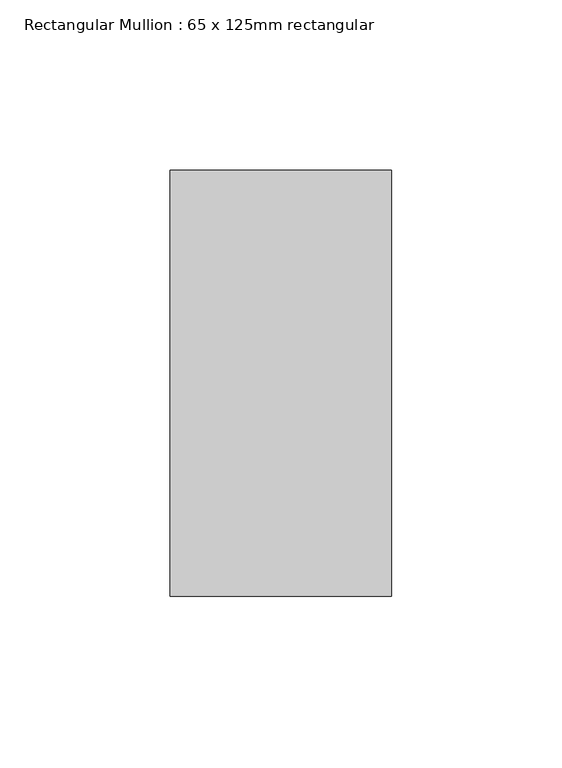
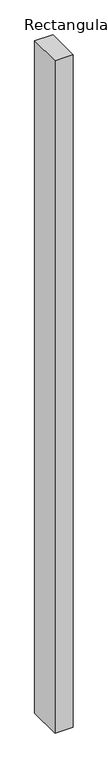
"""IFC4 building model written with IfcOpenShell, lengths in millimetres: member geometry, Rectangular Mullion : 65 x 125mm rectangular."""

from ifc_helpers import new_model, si_unit, frame, origin, place, context, project, spatial, polyline, outline, extrude, source, transform, mapped, element, save


def rectangular_mullion_65_x_125mm_rectangular_b6b0b808(model_context):
    return source(origin(), model_context, "Body", "SweptSolid", [
        extrude(outline(polyline([(0.0, 62.5), (0.0, -62.5), (-65.0, -62.5), (-65.0, 62.5), (0.0, 62.5)])), frame((0.0, 0.0, -2550.0), z_axis=(0.0, 0.0, 1.0), x_axis=(1.0, 0.0, 0.0)), (0.0, 0.0, 1.0), 2550.0),
    ])


if __name__ == "__main__":
    model = new_model("IFC4")
    model_context = context("Model", 3, world=origin())
    ifc_project = project(units=[si_unit("LENGTHUNIT", "METRE", prefix="MILLI")], contexts=[model_context])
    site = spatial("IfcSite", under=ifc_project)
    building = spatial("IfcBuilding", under=site)
    placement = place(None, origin())
    rectangular_mullion_65_x_125mm_rectangular_shape = rectangular_mullion_65_x_125mm_rectangular_b6b0b808(model_context)
    element("IfcMember", 1, ObjectType="Rectangular Mullion : 65 x 125mm rectangular", at=placement, inside=building, context=model_context, shape_type="MappedRepresentation", body=[
        mapped(rectangular_mullion_65_x_125mm_rectangular_shape, transform((0.0, 0.0, 0.0), x_axis=(1.0, 0.0, 0.0), y_axis=(0.0, 1.0, 0.0), z_axis=(0.0, 0.0, 1.0))),
    ])
    save(model, "model.ifc")

# Revit data of these elements
# Type "Rectangular Mullion : 65 x 125mm rectangular"
#   built-in parameter 1007304 = 0.410105 (stored number, unit not read)
#   built-in parameter 1007301 = 0.106627 (stored number, unit not read)
#   built-in parameter 1007300 = 0.106627 (stored number, unit not read)
# Element 1 (IfcMember, "Rectangular Mullion : 65 x 125mm rectangular")
#   Materials on its faces: "Aluminum"
# Materials
#   "Aluminum": class "Metal", colour RGB 244 245 246, transparency 0, Description = "Aluminum 6061", Cost = 0
